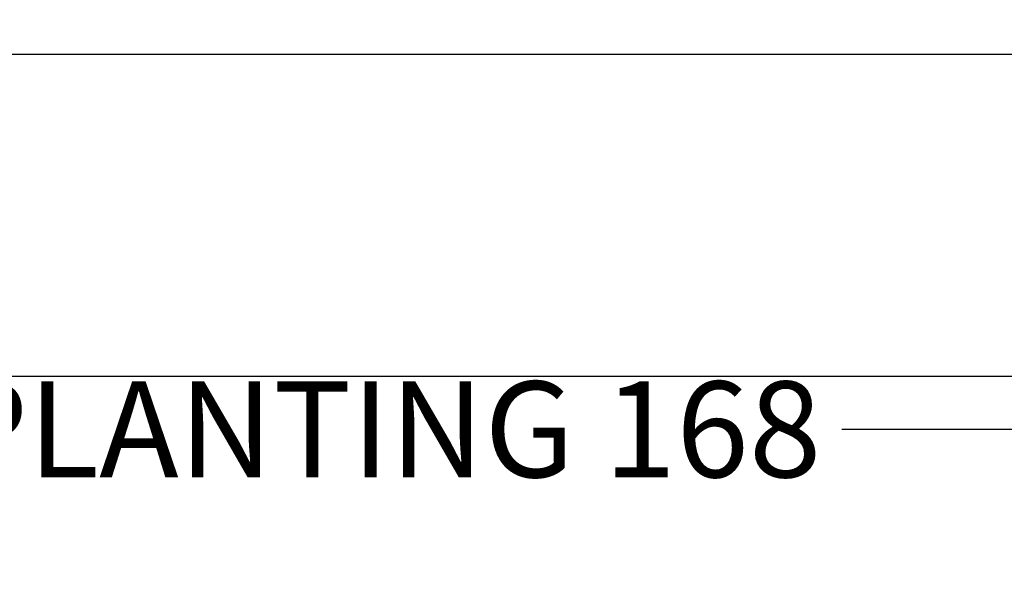
# Model space of a CAD drawing. Units: inches. Extents: x 89 to 490, y -59 to 378.
# Tile 8 of 20: x 339 to 400, y -59 to -24. Entities that reach past the tile are written whole.
import ezdxf

# ---------------------------------------------------------------- set-up
doc = ezdxf.new("R2010")
doc.units = ezdxf.units.IN
doc.header["$MEASUREMENT"] = 0
doc.layers.add('A-ANNO-DIMS', color=2, linetype='Continuous', lineweight=18)
doc.layers.add('L-PLNT-EDGE', color=31, linetype='Continuous', lineweight=25)
doc.styles.get("Standard").update_dxf_attribs({"font": 'arial.ttf'})
doc.dimstyles.get("Standard").update_dxf_attribs({"dimtxt": 6, "dimasz": 4, "dimexe": 3, "dimexo": 3, "dimgap": 0.09, "dimtad": 0, "dimtih": 1, "dimtoh": 1, "dimdec": 1, "dimzin": 0, "dimdsep": 46, "dimlunit": 3, "dimtxsty": 'Standard', "dimcen": 0.09, "dimadec": 0, "dimazin": 0, "dimtfac": 1, "dimtdec": 1, "dimtofl": 0, "dimtmove": 0, "dimatfit": 3, "dimfxl": 1, "dimtolj": 1, "dimtzin": 0, "dimarcsym": 0})

# ---------------------------------------------------------------- blocks, each defined once
blk = doc.blocks.new('*D46')
at = {"layer": 'A-ANNO-DIMS', "color": 0, "lineweight": -2, "transparency": 16777216}
for p, q in [((277.443, -27.866), (277.443, -53.11)), ((445.739, -27.866), (445.739, -53.11)), ((281.443, -50.11), (332.892, -50.11)), ((441.739, -50.11), (390.289, -50.11))]:
    blk.add_line(p, q, dxfattribs=at)
at = {"layer": 'A-ANNO-DIMS', "color": 0, "transparency": 16777216}
for points in [[(281.443, -49.443), (281.443, -50.777), (277.443, -50.11)], [(441.739, -49.443), (441.739, -50.777), (445.739, -50.11)]]:
    blk.add_solid(points, dxfattribs=at)
at = {"layer": 'Defpoints', "color": 0, "transparency": 16777216}
for p in [(277.443, -24.866), (445.739, -24.866), (445.739, -50.11)]:
    blk.add_point(p, dxfattribs=at)
at = {"layer": 'A-ANNO-DIMS', "color": 0, "transparency": 16777216, "insert": (361.591, -50.11), "char_height": 6, "attachment_point": 5}
blk.add_mtext('\\A1;PLANTING 168', dxfattribs=at)
blk = doc.blocks.new('*D48')
at = {"layer": 'A-ANNO-DIMS', "color": 0, "lineweight": -2, "transparency": 16777216}
for p, q in [((127.441, 10.741), (127.441, -49.809)), ((459.441, -29.659), (459.441, -49.809)), ((131.441, -46.809), (286.756, -46.809)), ((455.441, -46.809), (300.127, -46.809))]:
    blk.add_line(p, q, dxfattribs=at)
at = {"layer": 'A-ANNO-DIMS', "color": 0, "transparency": 16777216}
for points in [[(131.441, -46.143), (131.441, -47.476), (127.441, -46.809)], [(455.441, -46.143), (455.441, -47.476), (459.441, -46.809)]]:
    blk.add_solid(points, dxfattribs=at)
at = {"layer": 'Defpoints', "color": 0, "transparency": 16777216}
for p in [(127.441, 13.741), (459.441, -26.659), (459.441, -46.809)]:
    blk.add_point(p, dxfattribs=at)
at = {"layer": 'A-ANNO-DIMS', "color": 0, "transparency": 16777216, "insert": (293.441, -46.809), "char_height": 6, "attachment_point": 5}
blk.add_mtext('\\A1;332', dxfattribs=at)

msp = doc.modelspace()

# ---------------------------------------------------------------- linework, layer by layer
at = {"layer": 'L-PLNT-EDGE'}
msp.add_line((459.4414, -26.6594), (265.4414, -26.6594), dxfattribs=at)

# ---------------------------------------------------------------- dimensions: what is measured, and where the dimension line sits
at = {"layer": 'A-ANNO-DIMS'}
dim = msp.add_linear_dim(base=(459.4414, -46.8094), p1=(127.4414, 13.7413), p2=(459.4414, -26.6594), dimstyle='Standard', override={"dimdec": 0, "dimlfac": 1, "dimrnd": 0, "dimzin": 0, "dimdsep": 46, "dimlunit": 2}, dxfattribs=at)
dim.commit()
dim.dimension.update_dxf_attribs({"geometry": '*D48', "text_midpoint": (293.4414, -46.8094)})
dim = msp.add_linear_dim(base=(445.7386, -50.11), p1=(277.443, -24.8656), p2=(445.7386, -24.8656), text='PLANTING <>', dimstyle='Standard', override={"dimdec": 0, "dimlfac": 1, "dimrnd": 0, "dimzin": 0, "dimdsep": 46, "dimlunit": 2}, dxfattribs=at)
dim.commit()
dim.dimension.update_dxf_attribs({"geometry": '*D46', "text_midpoint": (361.5908, -50.11)})

doc.saveas('drawing.dxf')
